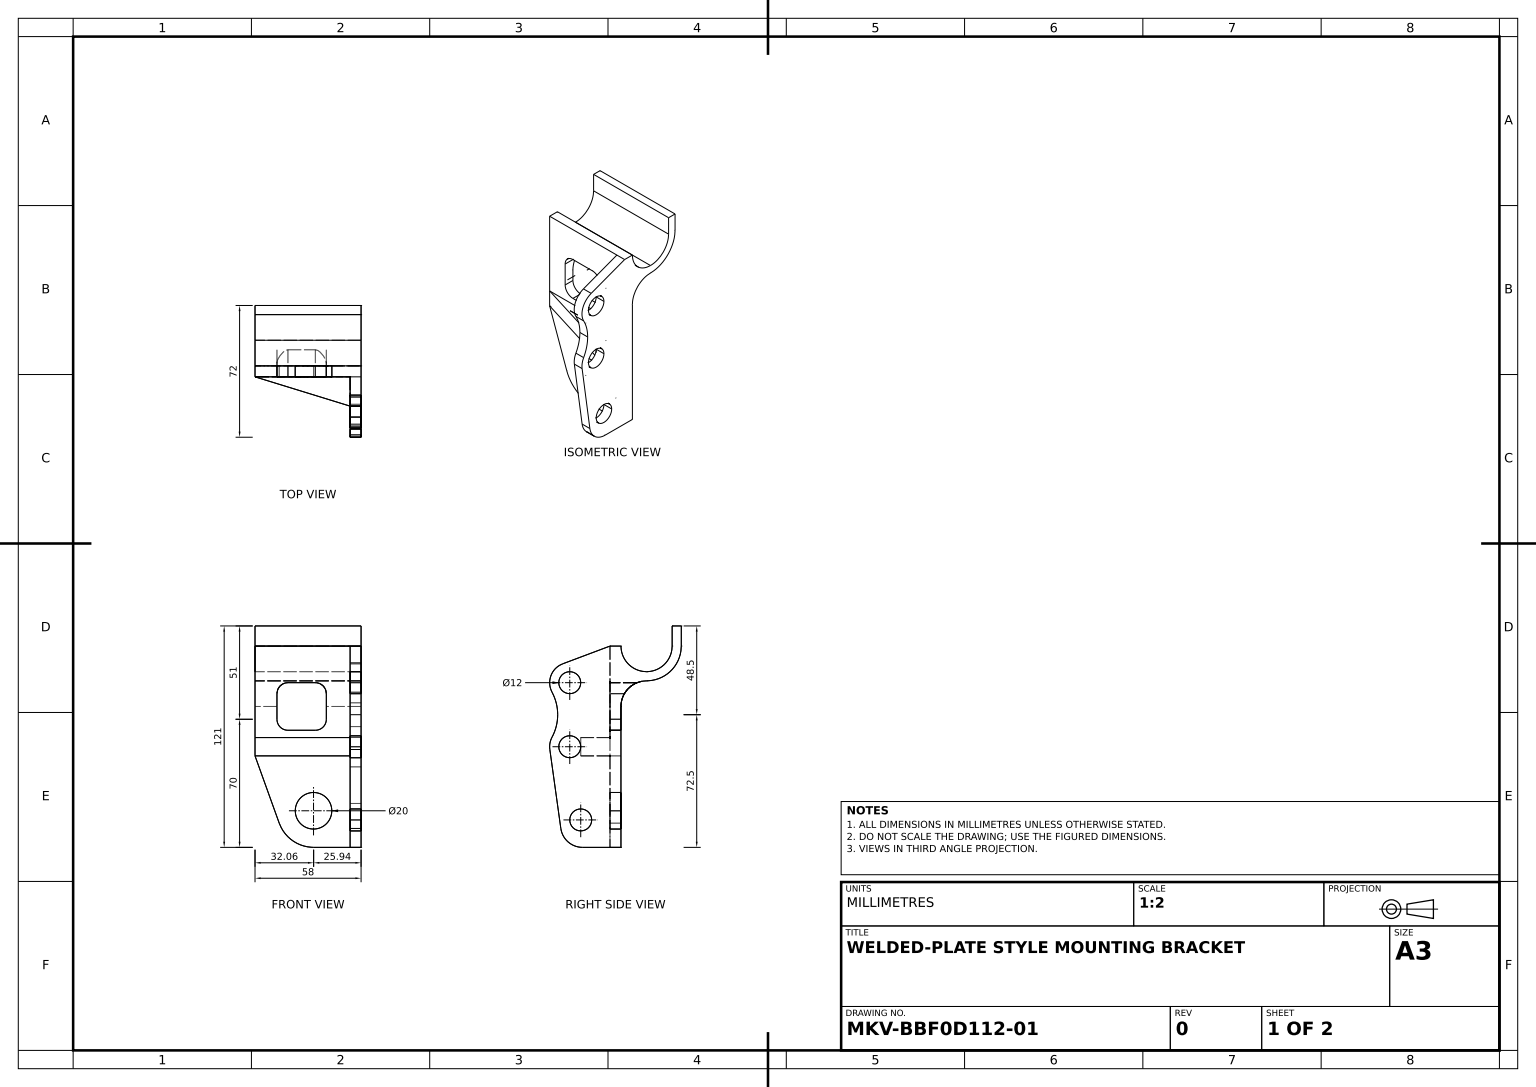
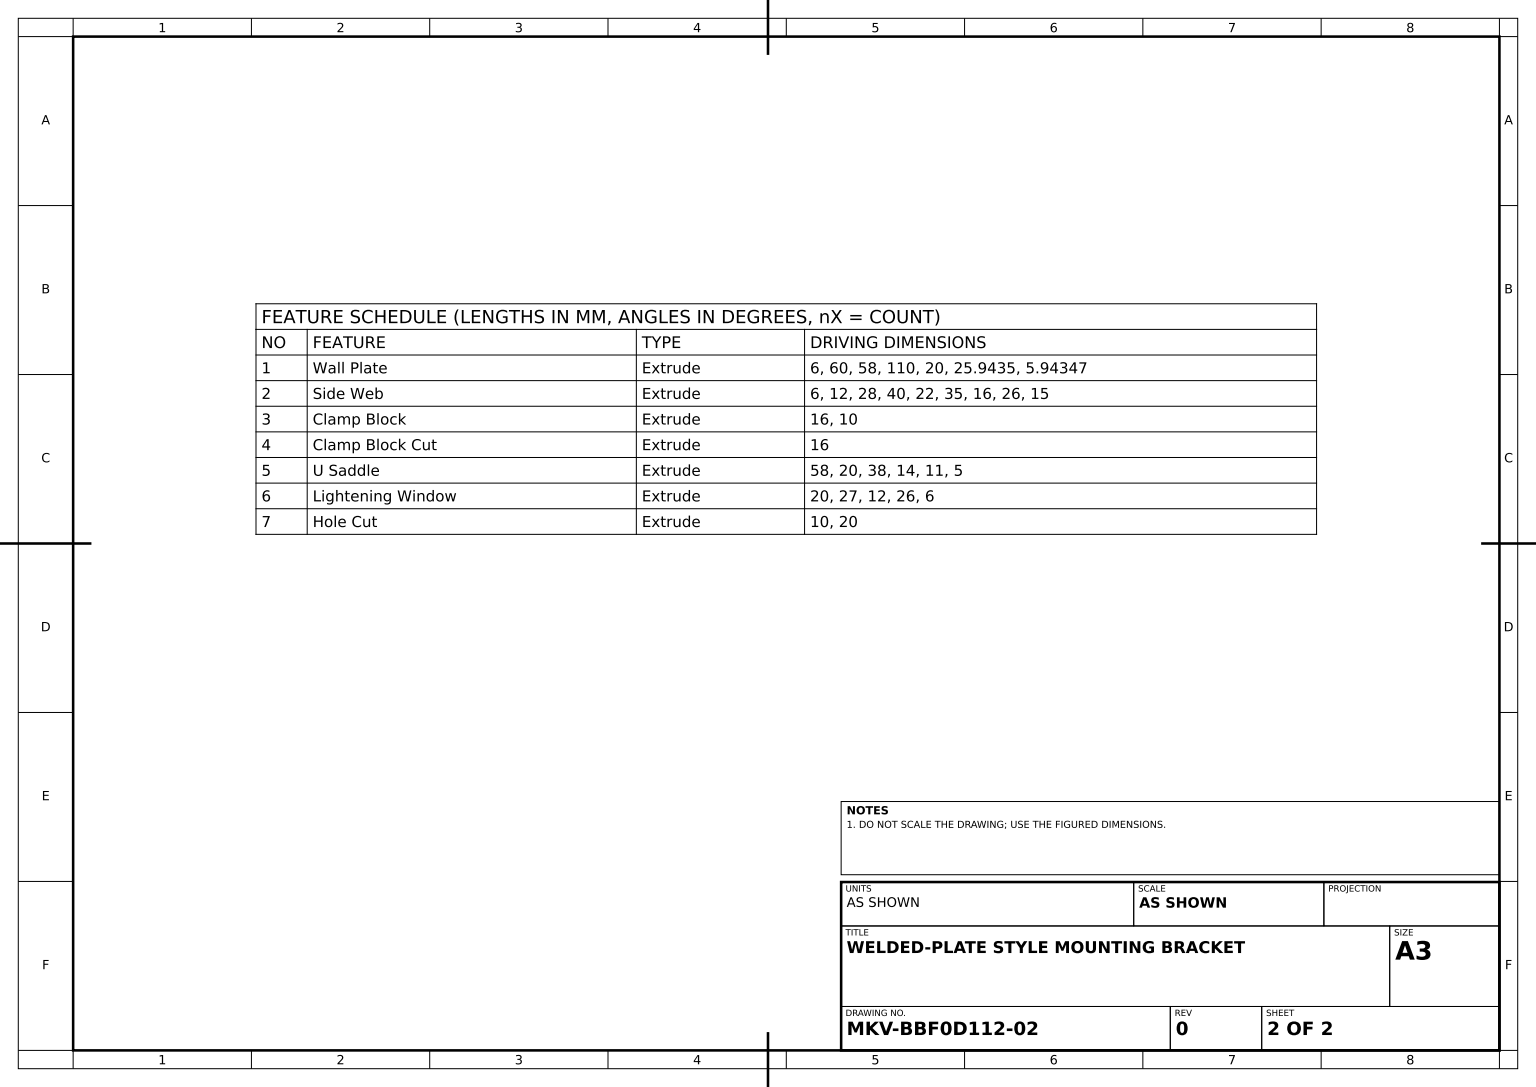
SolidWorks part; units mm, degrees
material "Plain Carbon Steel"
ref_plane "Front Plane" through (0, 0, 0) normal (0, 0, 1) x (1, 0, 0)
ref_plane "Top Plane" through (0, 0, 0) normal (0, 1, 0) x (1, 0, 0)
ref_plane "Right Plane" through (0, 0, 0) normal (1, 0, 0) x (0, 0, -1)
sketch "Wall Plate Sketch" plane through (0, 0, 0) normal (0, 0, 1) x (1, 0, 0)
  line L0 (0, 0) -> (0, -60)
  line L1 (0, 0) -> (58, 0)
  line L2 (58, 0) -> (58, -110)
  line L3 (58, -110) -> (38, -110)
  line L4 (38, -110) -> (32.0565, -110)
  line L5 (13.2388, -96.7744) -> (0, -60)
  arc A0 (32.0565, -110) -> (13.2388, -96.7744) centre (32.0565, -90) cw
  dimension "D4" = 20
  dimension "D1" = 60
  dimension "D2" = 58
  dimension "D3" = 110
  dimension "D5" = 25.9435
  dimension "D6" = 5.9435
extrude "Wall Plate" add sketch "Wall Plate Sketch" along normal blind 6
sketch "Side Web Sketch" plane through (58, 0, 0) normal (1, 0, 0) x (0, 0, -1)
  line L0 (0, -110) -> (0, 0) construction
  line L1 (-6, 0) -> (-31.8631, -9.7006)
  line L2 (-6, -110) -> (-6, 0) construction
  line L3 (-6, -110) -> (-21, -110)
  line L4 (-32.8852, -99.6557) -> (-38.8948, -56.5178)
  circle A0 centre (-28, -20) radius 6
  arc A1 (-31.8631, -9.7006) -> (-37.6918, -25.2027) centre (-28, -20) ccw
  circle A2 centre (-28, -55) radius 6
  arc A3 (-37.6918, -49.7973) -> (-38.8948, -56.5178) centre (-28, -55) ccw
  circle A4 centre (-22, -95) radius 6
  arc A5 (-37.6918, -25.2027) -> (-37.6918, -49.7973) centre (-60.5998, -37.5) cw
  arc A6 (-21, -110) -> (-32.8852, -99.6557) centre (-21, -98) cw
  line M6 (-6, 0) -> (-6, -110)
  dimension "D1" = 12
  dimension "D4" = 22
  dimension "D5" = 12
  dimension "D8" = 22
  dimension "D9" = 12
  dimension "D11" = 16
  dimension "D12" = 26
  dimension "D13" = 12
  dimension "D2" = 28
  dimension "D3" = 40
  dimension "D6" = 35
  dimension "D7" = 28
  dimension "D10" = 40
  dimension "D14" = 15
extrude "Side Web" add sketch "Side Web Sketch" against normal blind 6 contours A6 L3 L1 A1 A5 A3 L4 A4 A2 A0 M6
sketch "Clamp Block Sketch" plane through (0, 0, 6) normal (0, 0, 1) x (1, 0, 0)
  line L0 (52, -25.2027) -> (52, -49.7973) construction
  line L1 (0, -60) -> (52, -60)
  line L2 (0, -60) -> (0, -50)
  line L3 (0, -50) -> (52, -50)
  line L4 (52, -60) -> (52, -50)
  dimension "D1" = 10
extrude "Clamp Block" add sketch "Clamp Block Sketch" along normal blind 16
sketch "Clamp Block Cut Sketch" plane through (0, -50, 0) normal (0, 1, 0) x (1, 0, 0)
  line L0 (52, -22) -> (0, -6)
extrude "Clamp Block Cut" cut sketch "Clamp Block Cut Sketch" against normal blind 16 and the other way through all
sketch "U Saddle Sketch" plane through (0, 0, 0) normal (-1, 0, 0) x (0, 0, 1)
  line L0 (6, 0) -> (-14, 0) construction
  line L1 (0, 0) -> (0, -60) construction
  line L2 (-14, 0) -> (-28, 0) construction
  line L3 (0, 0) -> (0, -33)
  line L5 (-28, 0) -> (-28, 11)
  line L6 (-28, 11) -> (-33, 11)
  line L7 (-33, 0) -> (-33, 11)
  arc A0 (-28, 0) -> (0, 0) centre (-14, 0) ccw
  arc A1 (-33, 0) -> (-14, -19) centre (-14, 0) ccw
  arc A2 (-14, -19) -> (0, -33) centre (-14, -33) cw
  line M8 (0, 0) -> (0, -60)
  dimension "D2" = 38
  dimension "D3" = 14
  dimension "D1" = 20
  dimension "D4" = 11
  dimension "D5" = 5
  dimension "D6" = 11
extrude "U Saddle" add sketch "U Saddle Sketch" against normal blind 58 contours A1 A2 A0 L5 L6 L7 M8
sketch "Lightening Window Sketch" plane through (0, 0, 6) normal (0, 0, 1) x (1, 0, 0)
  line L0 (0, 0) -> (0, -50) construction
  line L1 (18, -20) -> (33, -20)
  line L2 (12, -26) -> (12, -40)
  line L3 (18, -46) -> (33, -46)
  line L4 (39, -26) -> (39, -40)
  line L5 (52, 0) -> (0, 0) construction
  arc A0 (33, -20) -> (39, -26) centre (33, -26) cw
  arc A1 (18, -20) -> (12, -26) centre (18, -26) ccw
  arc A2 (33, -46) -> (39, -40) centre (33, -40) ccw
  arc A3 (12, -40) -> (18, -46) centre (18, -40) ccw
  point P10 (39, -20)
  point P15 (39, -46)
  point P18 (12, -46)
  dimension "D5" = 6
  dimension "D1" = 27
  dimension "D2" = 12
  dimension "D3" = 26
  dimension "D4" = 20
extrude "Lightening Window" cut sketch "Lightening Window Sketch" against normal blind 20
sketch "Hole Sketch" plane through (0, 0, 6) normal (0, 0, 1) x (1, 0, 0)
  line L0 (52, -60) -> (52, -110) construction
  line L1 (32.0565, -110) -> (52, -110) construction
  circle A0 centre (32, -90) radius 10
  dimension "D1" = 20
  dimension "D2" = 20
  dimension "D3" = 20
extrude "Hole Cut" cut sketch "Hole Sketch" against normal blind 10
